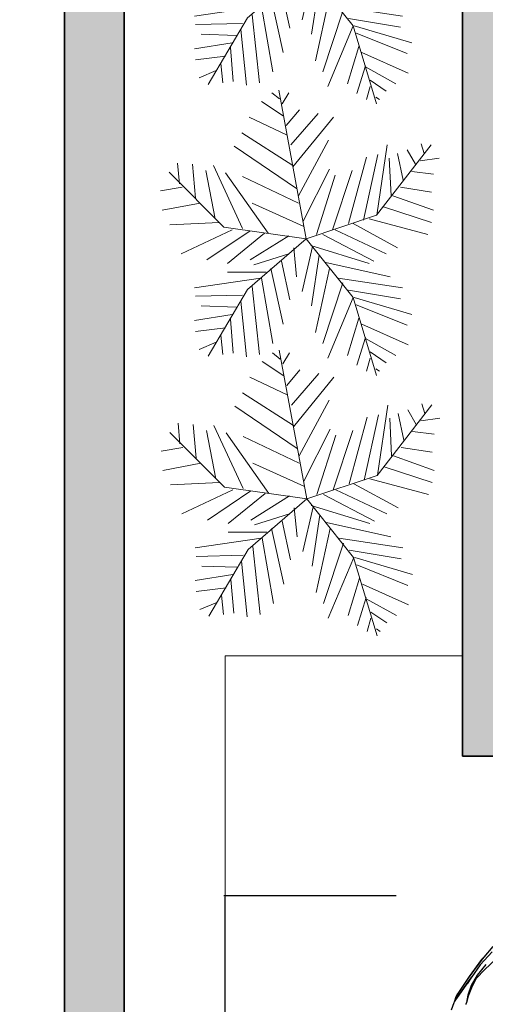
# Model space of a CAD drawing. Units: inches. Extents: x 1319 to 2030, y 219 to 1069.
# Tile 16 of 28: x 1363 to 1433, y 515 to 663. Entities that reach past the tile are written whole.
import ezdxf

# ---------------------------------------------------------------- set-up
doc = ezdxf.new("R2010")
doc.units = ezdxf.units.IN
doc.header["$MEASUREMENT"] = 0
doc.layers.get('0').update_dxf_attribs({"color": 12})
for name, color, linetype, lineweight in [('A-ANNO-DIMS', 2, 'Continuous', 18), ('A-FLOR', 8, 'Continuous', 18), ('A-WALL-PATT', 252, 'Continuous', 13), ('C-PRKG-VEHC', 8, 'Continuous', 13), ('C-PROP', 7, 'Continuous', 35), ('lawn', 82, 'Continuous', 13), ('walls', 250, 'Continuous', 35)]:
    doc.layers.add(name, color=color, linetype=linetype, lineweight=lineweight)
doc.layers.add('Edges', color=250, linetype='Continuous')
doc.styles.get("Standard").update_dxf_attribs({"font": 'arial.ttf'})
doc.dimstyles.get("Standard").update_dxf_attribs({"dimtxt": 7, "dimasz": 0.18, "dimexe": 0.18, "dimexo": 0.0625, "dimgap": 0.09, "dimtad": 0, "dimtih": 1, "dimtoh": 1, "dimzin": 0, "dimdsep": 46, "dimlunit": 3, "dimtxsty": 'Standard', "dimcen": 0.09, "dimadec": 0, "dimazin": 0, "dimtfac": 1, "dimtofl": 0, "dimtmove": 0, "dimatfit": 3, "dimfxl": 1, "dimtolj": 1, "dimtzin": 0, "dimarcsym": 0})

# ---------------------------------------------------------------- blocks, each defined once
blk = doc.blocks.new('Nissan Qashqai pl')
at = {"layer": 'Edges'}
for p, q in [((7.4801, 11.2168), (7.5217, 11.1823)), ((7.5001, 11.2139), (7.5501, 11.1684)), ((7.5289, 11.2283), (7.5687, 11.1862)), ((7.5304, 11.1737), (7.5217, 11.1823)), ((7.5217, 11.1823), (7.5387, 11.1682)), ((7.5304, 11.1737), (7.5946, 11.1262)), ((7.5387, 11.1682), (7.6031, 11.1217)), ((7.5492, 11.1902), (7.59, 11.1565)), ((7.5501, 11.1684), (7.5969, 11.1365)), ((7.5687, 11.1862), (7.6032, 11.1533)), ((7.59, 11.1565), (7.6295, 11.1344)), ((7.6113, 11.1256), (7.5969, 11.1365)), ((7.5969, 11.1365), (7.6021, 11.1329)), ((7.6021, 11.1329), (7.6118, 11.1255)), ((7.6021, 11.1329), (7.6237, 11.1181)), ((7.6032, 11.1533), (7.6386, 11.1353)), ((7.6295, 11.1344), (7.667, 11.1212)), ((7.6386, 11.1353), (7.6708, 11.1225)), ((7.5946, 11.1262), (7.6608, 11.0825)), ((7.6676, 11.0791), (7.6024, 11.1221)), ((7.6759, 11.0809), (7.6113, 11.1256)), ((7.6118, 11.1255), (7.6799, 11.0783)), ((7.667, 11.1212), (7.6949, 11.1158)), ((7.6708, 11.1225), (7.6949, 11.1158)), ((7.6949, 11.1158), (7.701, 11.1141)), ((7.701, 11.1141), (7.7024, 11.1141)), ((7.6712, 11.0767), (7.6608, 11.0825)), ((7.6721, 11.0762), (7.6712, 11.0767)), ((7.6926, 11.0705), (7.6721, 11.0762)), ((7.6793, 11.0784), (7.6759, 11.0809)), ((7.6802, 11.0782), (7.6793, 11.0784)), ((7.6802, 11.0782), (7.6799, 11.0783)), ((7.6809, 11.0777), (7.6802, 11.0782)), ((7.6926, 11.0705), (7.6809, 11.0777)), ((7.6953, 11.0688), (7.6926, 11.0705)), ((7.7223, 11.059), (7.6953, 11.0688))]:
    blk.add_line(p, q, dxfattribs=at)
blk = doc.blocks.new('car')
blk.add_blockref('Nissan Qashqai pl', (-9.7433, -11.9151))
blk = doc.blocks.new('carr')
blk.add_blockref('car', (0.5124, -0.007))
blk = doc.blocks.new('*U27')
for p, q in [((0, 0), (-10.5, 57)), ((-10.186, 53.64), (-13.084, 55.962)), ((-9.099, 51.782), (-6.563, 55.962)), ((-8.737, 47.138), (-17.069, 52.711)), ((-7.65, 43.423), (-2.578, 49.46)), ((-7.288, 39.707), (-21.778, 46.673)), ((-5.839, 35.992), (4.667, 48.067)), ((-5.114, 27.632), (10.463, 46.673)), ((-5.114, 28.097), (-24.676, 40.636)), ((-2.941, 16.486), (8.652, 37.85)), ((-3.665, 19.273), (-27.574, 35.527)), ((27, 9), (48, 36)), ((27.127, 9.056), (31.112, 35.992)), ((38.719, 34.134), (41.979, 28.561)), ((44.153, 36.456), (45.239, 32.741)), ((16.259, 5.805), (23.142, 31.348)), ((22.055, 7.198), (27.489, 32.277)), ((31.836, 30.883), (32.561, 16.486)), ((35.096, 32.741), (37.27, 22.524)), ((43.791, 29.954), (51.036, 30.883)), ((-48.585, 21.131), (-49.309, 29.026)), ((-43.513, 28.561), (-42.427, 15.558)), ((-35.544, 28.097), (-24.314, 3.947)), ((-1.129, 6.734), (9.014, 26.704)), ((-31.5, 4.5), (-52.5, 25.5)), ((-38.442, 26.239), (-34.819, 7.663)), ((-14.533, 2.09), (-30.834, 25.31)), ((-24.314, 23.917), (-2.941, 13.7)), ((3.942, 1.625), (11.187, 24.381)), ((10.101, 3.483), (17.708, 26.239)), ((40.53, 25.775), (48.862, 24.846)), ((-47.498, 19.737), (-55.83, 18.344)), ((36.183, 19.737), (48.137, 17.88)), ((33.285, 16.486), (48.862, 10.913)), ((-40.615, 13.7), (-55.105, 10.913)), ((-20.691, 13.7), (-1.129, 4.876)), ((29.662, 12.307), (48.137, 6.269)), ((0, 0), (27, 9)), ((24.229, 7.663), (46.688, 1.625)), ((-33.37, 6.269), (-52.207, 5.34)), ((0, 0), (-31.5, 4.5)), ((18.07, 5.805), (35.096, -3.483)), ((-28.299, 3.483), (-47.86, -5.805)), ((-21.416, 3.018), (-38.079, -8.128)), ((-15.982, 2.09), (-30.11, -9.521)), ((0, 0), (-22.5, -19.5)), ((-6.563, 1.161), (-21.416, -8.128)), ((0, 0), (18, -22.5)), ((6.478, 1.625), (26.04, -8.592)), ((11.187, 3.483), (30.749, -5.805)), ((-4.752, -3.483), (-3.665, -14.629)), ((2.493, -3.019), (-1.491, -20.202)), ((1.769, -2.555), (24.229, -9.521)), ((-6.563, -5.805), (-19.967, -9.985)), ((5.029, -6.27), (2.131, -25.775)), ((-9.461, -8.592), (-6.201, -23.453)), ((7.565, -9.056), (32.198, -14.629)), ((-17.431, -15.094), (-42.789, -18.809)), ((-15.257, -12.772), (-30.11, -12.772)), ((-17.069, -15.094), (-12.721, -40.172)), ((-13.446, -11.378), (-8.737, -32.741)), ((9.014, -11.378), (3.58, -35.992)), ((12.274, -15.094), (36.907, -18.809)), ((-20.691, -18.345), (-17.793, -44.352)), ((14.085, -16.951), (6.478, -40.172)), ((-24.314, -21.596), (-42.427, -22.06)), ((-22.5, -19.5), (-37.5, -45)), ((18.07, -22.524), (8.289, -45.745)), ((16.259, -19.738), (36.183, -22.989)), ((18, -22.5), (27, -52.5)), ((18.433, -22.524), (40.53, -29.026)), ((-26.849, -26.24), (-40.253, -25.775)), ((-25.038, -23.918), (-22.865, -45.281)), ((19.157, -25.311), (38.719, -33.206)), ((-28.299, -29.026), (-42.789, -31.348)), ((-29.023, -30.884), (-27.936, -43.887)), ((20.244, -30.419), (15.897, -44.816)), ((21.331, -32.741), (39.081, -40.636)), ((-30.834, -34.135), (-42.427, -35.528)), ((-32.646, -36.921), (-31.921, -44.352)), ((-34.457, -39.708), (-40.978, -42.494)), ((22.78, -37.85), (19.519, -48.532)), ((22.78, -38.314), (34.372, -44.816)), ((24.591, -43.423), (30.749, -47.603)), ((24.591, -45.745), (23.142, -50.854)), ((26.764, -49.925), (28.213, -50.854))]:
    blk.add_line(p, q)
blk = doc.blocks.new('*D56')
at = {"layer": 'A-ANNO-DIMS', "color": 0, "lineweight": -2, "transparency": 16777216}
for p, q in [((1419.85, 531.2), (1393.86, 531.2)), ((1394.04, 531.02), (1394.04, 448.68)), ((1394.04, 358.92), (1394.04, 441.26)), ((1419.85, 358.74), (1393.86, 358.74))]:
    blk.add_line(p, q, dxfattribs=at)
at = {"layer": 'A-ANNO-DIMS', "color": 0, "transparency": 16777216}
for points in [[(1394.01, 531.02), (1394.07, 531.02), (1394.04, 531.2)], [(1394.01, 358.92), (1394.07, 358.92), (1394.04, 358.74)]]:
    blk.add_solid(points, dxfattribs=at)
at = {"layer": 'Defpoints', "color": 0, "transparency": 16777216}
for p in [(1419.91, 531.2), (1394.04, 358.74), (1419.91, 358.74)]:
    blk.add_point(p, dxfattribs=at)
at = {"layer": 'A-ANNO-DIMS', "color": 0, "transparency": 16777216, "insert": (1394.04, 444.97), "char_height": 7, "attachment_point": 5}
blk.add_mtext('\\A1;CAR 14\'-4 1/2"', dxfattribs=at)

msp = doc.modelspace()

# ---------------------------------------------------------------- hatches: boundary and pattern name
at = {"layer": 'A-WALL-PATT'}
h = msp.add_hatch(color=256, dxfattribs=at)
h.dxf.hatch_style = 1
h.paths.add_polyline_path([(1378.843, 946.227), (1960.843, 946.227), (1960.843, 860.616), (1922.194, 860.616), (1922.194, 851.616), (1960.843, 851.616), (1960.843, 304.227), (1578.343, 304.227), (1578.343, 295.227), (1969.843, 295.227), (1969.843, 955.227), (1369.843, 955.227), (1369.843, 295.227), (1378.843, 295.227)])
h = msp.add_hatch(color=256, dxfattribs=at)
h.dxf.hatch_style = 1
h.paths.add_polyline_path([(1856.292, 860.616), (1812.343, 860.616), (1812.343, 851.616), (1812.343, 700.993), (1816.843, 700.993), (1816.843, 851.616), (1856.292, 851.616)])
h.paths.add_polyline_path([(1960.843, 663.616), (1812.343, 663.616), (1782.783, 663.616), (1782.783, 659.116), (1812.343, 659.116), (1960.843, 659.116)])
h.paths.add_polyline_path([(1857.424, 659.116), (1852.924, 659.116), (1852.924, 616.807), (1857.424, 616.807)])
h.paths.add_polyline_path([(1735.843, 661.727), (1731.843, 661.727), (1636.133, 661.727), (1636.133, 657.227), (1731.343, 657.227), (1731.343, 481.227), (1618.616, 481.227), (1618.616, 472.227), (1639.343, 472.227), (1639.343, 384.227), (1627.044, 384.227), (1627.044, 375.227), (1648.343, 375.227), (1648.343, 384.227), (1648.343, 472.227), (1750.706, 472.227), (1750.706, 481.227), (1735.843, 481.227), (1735.843, 657.727)])
h.paths.add_polyline_path([(1587.343, 481.227), (1578.343, 481.227), (1578.343, 375.227), (1597.622, 375.227), (1597.622, 384.227), (1587.343, 384.227)])
h.paths.add_polyline_path([(1769.593, 384.227), (1693.482, 384.227), (1693.482, 375.227), (1769.593, 375.227)])
h.paths.add_polyline_path([(1775.828, 481.227), (1765.831, 481.227), (1765.831, 472.227), (1775.828, 472.227)])
h.paths.add_polyline_path([(1824.625, 481.227), (1820.343, 481.227), (1820.343, 476.727), (1824.625, 476.727), (1824.625, 477.545)], flags=0)
h.paths.add_polyline_path([(1896.843, 481.227), (1852.26, 481.227), (1852.26, 476.727), (1892.343, 476.727), (1892.343, 384.227), (1881.742, 384.227), (1881.742, 375.227), (1913.435, 375.227), (1913.435, 384.227), (1896.843, 384.227)])
h.paths.add_polyline_path([(1960.843, 481.227), (1931.341, 481.227), (1931.341, 476.727), (1960.843, 476.727)])
h.paths.add_polyline_path([(1736.343, 918.227), (1731.843, 918.227), (1731.843, 890.227), (1582.843, 890.227), (1582.843, 781.727), (1582.843, 769.171), (1587.343, 769.171), (1587.343, 781.727), (1587.343, 885.727), (1731.843, 885.727), (1731.843, 851.616), (1736.343, 851.616), (1736.343, 890.227)])
h.paths.add_polyline_path([(1781.022, 860.616), (1773.021, 860.616, -0.0322281), (1773.289, 856.464), (1773.289, 851.616), (1781.022, 851.616)])
h.paths.add_polyline_path([(1587.343, 946.227), (1582.843, 946.227), (1582.843, 926.136), (1587.343, 926.136)])
h.paths.add_polyline_path([(1647.843, 946.227), (1643.343, 946.227), (1643.343, 926.136), (1647.843, 926.136)])
h.paths.add_polyline_path([(1543.343, 786.227), (1429.843, 786.227), (1429.843, 757.555), (1434.343, 757.555), (1438.843, 757.555), (1438.843, 781.727), (1543.343, 781.727)])
h.paths.add_polyline_path([(1543.343, 781.727), (1538.843, 781.727), (1538.843, 709.727), (1534.597, 709.727), (1534.597, 705.227), (1543.343, 705.227), (1543.343, 709.727)])
h.paths.add_polyline_path([(1499.955, 709.727), (1438.843, 709.727), (1438.843, 734.463), (1429.843, 734.463), (1429.843, 552.227), (1470.241, 552.227), (1470.241, 561.227), (1438.843, 561.227), (1438.843, 705.227), (1499.955, 705.227)])
h.paths.add_polyline_path([(1587.343, 709.727), (1582.843, 709.727), (1582.843, 561.227), (1543.433, 561.227), (1543.433, 552.227), (1587.343, 552.227)])
h.paths.add_polyline_path([(1546.835, 709.727), (1543.343, 709.727), (1543.343, 705.227), (1546.835, 705.227)])
h.paths.add_polyline_path([(1582.843, 709.727), (1579.15, 709.727), (1579.15, 705.227), (1582.843, 705.227)], flags=17)
h.paths.add_polyline_path([(1548.368, 786.227), (1543.343, 786.227), (1543.343, 781.727), (1548.368, 781.727)])
h.paths.add_polyline_path([(1582.843, 786.227), (1580.683, 786.227), (1580.683, 781.727), (1582.843, 781.727)])
h.paths.add_polyline_path([(1587.343, 892.402), (1582.843, 892.402), (1582.843, 890.227), (1587.343, 890.227)], flags=17)
h.paths.add_polyline_path([(1647.843, 892.402), (1643.343, 892.402), (1643.343, 890.227), (1647.843, 890.227)], flags=17)
h.paths.add_polyline_path([(1740.974, 856.464), (1740.974, 860.616), (1736.343, 860.616), (1736.343, 851.616), (1740.974, 851.616)])
h.paths.add_polyline_path([(1853.989, 384.227), (1820.343, 384.227), (1820.343, 402.924), (1815.843, 402.924), (1815.843, 375.227), (1853.989, 375.227)])
h.paths.add_polyline_path([(1892.343, 436.227), (1820.343, 436.227), (1820.343, 481.227), (1815.843, 481.227), (1815.843, 431.727), (1892.343, 431.727)])
h.paths.add_polyline_path([(1849.175, 481.227), (1824.625, 481.227), (1824.625, 477.545), (1825.699, 477.545), (1825.699, 453.018, 0.4014527), (1849.175, 477.545)], flags=0)
h.paths.add_polyline_path([(1960.843, 384.227), (1941.188, 384.227), (1941.188, 375.227), (1960.843, 375.227)])
h.paths.add_polyline_path([(1902.267, 481.227), (1896.843, 481.227), (1896.843, 476.727), (1902.267, 476.727), (1902.267, 477.44)], flags=0)

# ---------------------------------------------------------------- linework, layer by layer
at = {"layer": 'A-FLOR'}
for p, q in [((1429.843, 567.372), (1394.092, 567.372)), ((1394.092, 567.372), (1394.092, 337.406))]:
    msp.add_line(p, q, dxfattribs=at)
at = {"layer": 'C-PROP'}
msp.add_line((1369.843, 295.227), (1369.843, 955.227), dxfattribs=at)
at = {"layer": 'walls'}
for p, q in [((1378.843, 295.227), (1378.843, 946.227)), ((1429.843, 552.227), (1429.843, 786.227)), ((1429.843, 552.227), (1587.343, 552.227))]:
    msp.add_line(p, q, dxfattribs=at)

# ---------------------------------------------------------------- block references
at = {"layer": 'C-PRKG-VEHC', "xscale": 39.37007874015748, "yscale": 39.37007874015748, "zscale": 39.37007874015748, "rotation": 270}
msp.add_blockref('carr', (1462.179, 454.621), dxfattribs=at)
at = {"layer": 'lawn', "xscale": 0.39313680782538, "yscale": 0.39313680782538, "zscale": 0.39313680782538}
for p in [(1406.267, 671.257), (1406.267, 630.284), (1406.363, 591.061)]:
    msp.add_blockref('*U27', p, dxfattribs=at)

# ---------------------------------------------------------------- dimensions: what is measured, and where the dimension line sits
at = {"layer": 'A-ANNO-DIMS'}
dim = msp.add_linear_dim(base=(1394.045, 358.738), p1=(1419.914, 531.201), p2=(1419.914, 358.738), angle=270, text='CAR <>', dimstyle='Standard', override={"dimdec": 1, "dimlfac": 1, "dimrnd": 0, "dimzin": 1, "dimdsep": 46, "dimlunit": 4, "dimfrac": 2}, dxfattribs=at)
dim.commit()
dim.dimension.update_dxf_attribs({"geometry": '*D56', "text_midpoint": (1394.045, 444.969)})

doc.saveas('drawing.dxf')
